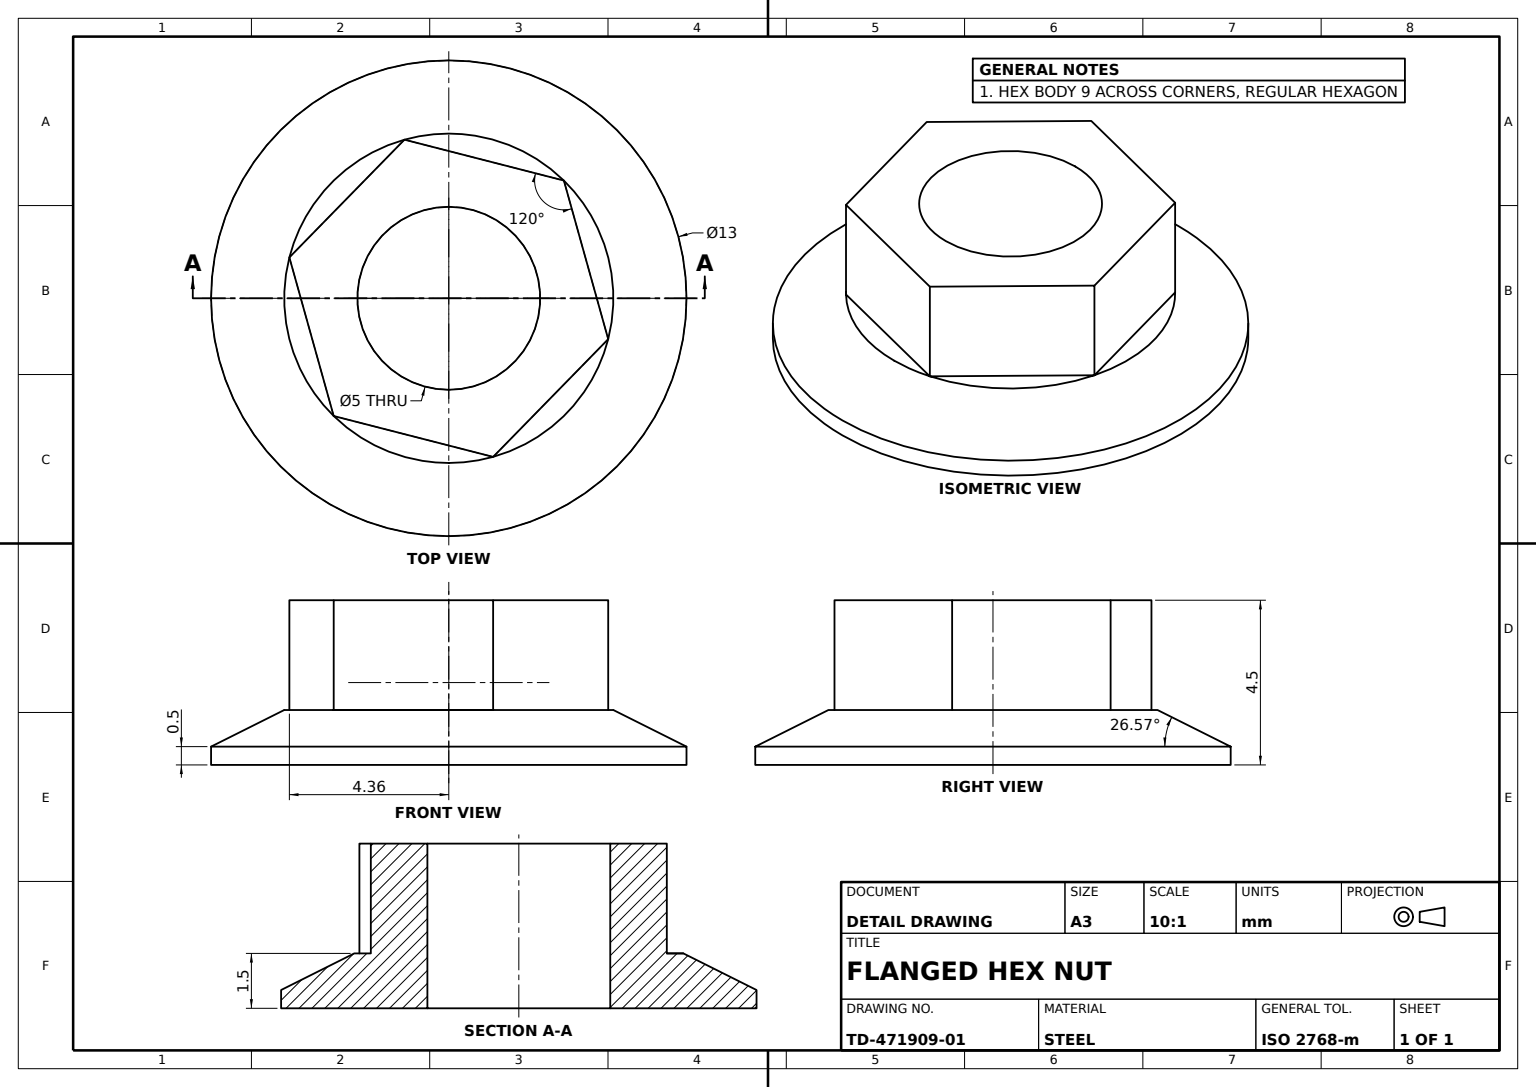
from build123d import *

# Parameters (mm, degrees)
NUT_PROFILE_SKETCH_R     = 6.5
FLANGE_DISC_13_DEPTH     = 0.5
SKETCH1_5_R              = 4.5
FLANGE_COLLAR_DEPTH      = 1.5
SKETCH1_6_R              = 2.5
HEX_BODY_DEPTH           = 4.5
TAPER_LOFT_BASE_SKETCH_R = 6.5
TAPER_LOFT_TOP_SKETCH_R  = 4.5
THROUGH_START            = -4.5
BORE_SKETCH_R            = 2.5
THROUGH_BORE_DEPTH       = 4.5


with BuildPart() as part:
    # Nut Profile Sketch → Flange Disc _13 (new body)
    with BuildSketch(Plane(origin=(0, 0, 0), x_dir=(1, 0, 0), z_dir=(0, 1, 0))):
        with Locations(Location((0, 0, 0), (0, 0, 270))):
            Circle(NUT_PROFILE_SKETCH_R)
    extrude(amount=FLANGE_DISC_13_DEPTH)

    # Sketch1_5 → Flange Collar (add)
    with BuildSketch(Plane(origin=(0, 0, 0), x_dir=(1, 0, 0), z_dir=(0, 1, 0))):
        with Locations(Location((0, 0, 0), (0, 0, 270))):
            Circle(SKETCH1_5_R)
    extrude(amount=FLANGE_COLLAR_DEPTH)

    # Sketch1_6 → Hex Body (add)
    with BuildSketch(Plane(origin=(0, 0, 0), x_dir=(1, 0, 0), z_dir=(0, 1, 0))):
        Polygon((-3.14677035, -3.216805304), (1.212449938, -4.333585715), (4.359220287, -1.116780411), (3.14677035, 3.216805304), (-1.212449938, 4.333585715), (-4.359220287, 1.116780411), align=None)
        with Locations(Location((0, 0, 0), (0, 0, 270))):
            Circle(SKETCH1_6_R, mode=Mode.SUBTRACT)
    extrude(amount=HEX_BODY_DEPTH)

    # Taper Loft Base Sketch → Flange Taper Loft section 0
    with BuildSketch(Plane(origin=(0, 0.5, 0), x_dir=(1, 0, 0), z_dir=(0, 1, 0))):
        Circle(TAPER_LOFT_BASE_SKETCH_R)
    # Taper Loft Top Sketch → Flange Taper Loft section 1
    with BuildSketch(Plane(origin=(0, 1.5, 0), x_dir=(1, 0, 0), z_dir=(0, 1, 0))):
        Circle(TAPER_LOFT_TOP_SKETCH_R)
    loft()

    # Bore Sketch → Through Bore (cut)
    with BuildSketch(Plane(origin=(0, 1.5, 0), x_dir=(1, 0, 0), z_dir=(0, 1, 0)).offset(THROUGH_START)):
        with Locations(Location((0, 0, 0), (0, 0, 270))):
            Circle(BORE_SKETCH_R)
    extrude(amount=THROUGH_BORE_DEPTH, mode=Mode.SUBTRACT)


solid = part.part
